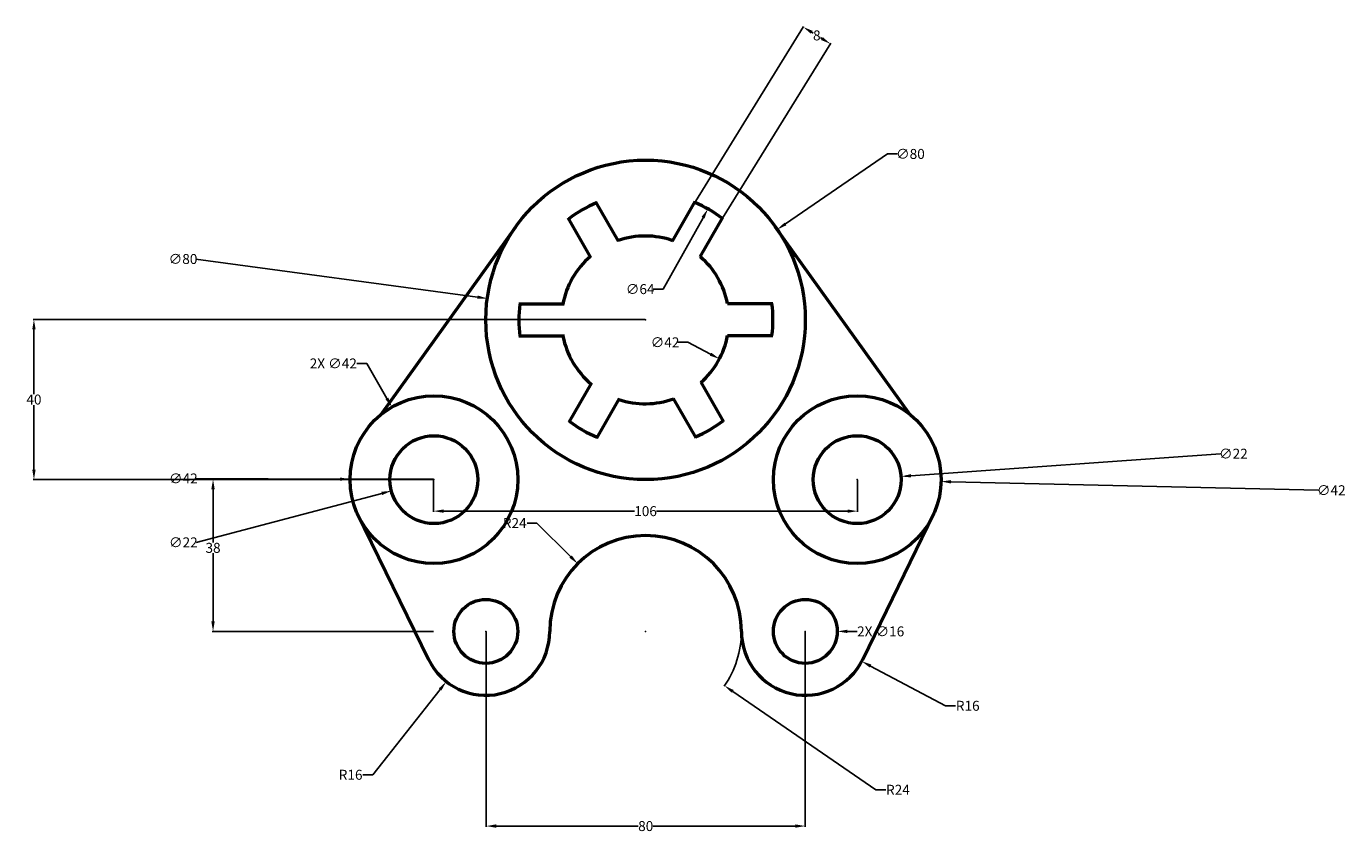
# Model space of a CAD drawing. Units: millimetres. Extents: x -109 to 221, y -17 to 185.
import ezdxf

# ---------------------------------------------------------------- set-up
doc = ezdxf.new("R2010")
doc.units = ezdxf.units.MM
doc.header["$MEASUREMENT"] = 0
doc.linetypes.add('CENTER', pattern=[50.8, 31.75, -6.35, 6.35, -6.35])
for name, color, linetype, lineweight in [('M-CNTR', 1, 'CENTER', 18), ('M-DIMS', 2, 'Continuous', 25), ('M-OUTL', 7, 'Continuous', 50)]:
    doc.layers.add(name, color=color, linetype=linetype, lineweight=lineweight)
doc.styles.get("Standard").update_dxf_attribs({"font": 'arial.ttf'})
doc.dimstyles.get("Standard").update_dxf_attribs({"dimtxt": 2.5, "dimasz": 2.5, "dimexe": 0.18, "dimexo": 0.0625, "dimgap": 0.09, "dimtad": 0, "dimtih": 1, "dimtoh": 1, "dimdec": 0, "dimzin": 0, "dimdsep": 46, "dimtxsty": 'Standard', "dimcen": 0.09, "dimadec": 0, "dimazin": 0, "dimtfac": 1, "dimtdec": 0, "dimtofl": 0, "dimtmove": 0, "dimatfit": 3, "dimfxl": 1, "dimtolj": 1, "dimtzin": 0, "dimarcsym": 0})

# ---------------------------------------------------------------- blocks, each defined once
blk = doc.blocks.new('*D1')
at = {"layer": 'Defpoints', "color": 0, "transparency": 16777216}
for p in [(5.99, 117.08), (85.26, 106.35)]:
    blk.add_point(p, dxfattribs=at)
at = {"layer": 'M-DIMS', "color": 0, "lineweight": -2, "transparency": 16777216}
for p, q in [((-66.97, 126.95), (3.51, 117.41)), ((45.54, 111.71), (45.72, 111.71)), ((45.63, 111.62), (45.63, 111.8))]:
    blk.add_line(p, q, dxfattribs=at)
at = {"layer": 'M-DIMS', "color": 0, "transparency": 16777216}
blk.add_solid([(3.57, 117.82), (3.45, 117), (5.99, 117.08)], dxfattribs=at)
at = {"layer": 'M-DIMS', "color": 0, "transparency": 16777216, "insert": (-70.2, 126.95), "char_height": 2.5, "attachment_point": 5}
blk.add_mtext('\\A1;∅80', dxfattribs=at)
blk = doc.blocks.new('*D2')
at = {"layer": 'Defpoints', "color": 0, "transparency": 16777216}
for p in [(-28.37, 71.82), (13.63, 71.61)]:
    blk.add_point(p, dxfattribs=at)
at = {"layer": 'M-DIMS', "color": 0, "lineweight": -2, "transparency": 16777216}
for p, q in [((-66.89, 72), (-30.87, 71.83)), ((-7.46, 71.71), (-7.28, 71.71)), ((-7.37, 71.62), (-7.37, 71.8))]:
    blk.add_line(p, q, dxfattribs=at)
at = {"layer": 'M-DIMS', "color": 0, "transparency": 16777216}
blk.add_solid([(-30.87, 72.24), (-30.88, 71.41), (-28.37, 71.82)], dxfattribs=at)
at = {"layer": 'M-DIMS', "color": 0, "transparency": 16777216, "insert": (-70.12, 72), "char_height": 2.5, "attachment_point": 5}
blk.add_mtext('\\A1;∅42', dxfattribs=at)
blk = doc.blocks.new('*D3')
at = {"layer": 'Defpoints', "color": 0, "transparency": 16777216}
for p in [(3.26, 74.52), (-18.01, 68.9)]:
    blk.add_point(p, dxfattribs=at)
at = {"layer": 'M-DIMS', "color": 0, "lineweight": -2, "transparency": 16777216}
for p, q in [((-7.46, 71.71), (-7.28, 71.71)), ((-7.37, 71.62), (-7.37, 71.8)), ((-66.89, 56), (-20.43, 68.27))]:
    blk.add_line(p, q, dxfattribs=at)
at = {"layer": 'M-DIMS', "color": 0, "transparency": 16777216}
blk.add_solid([(-20.53, 68.67), (-20.32, 67.86), (-18.01, 68.9)], dxfattribs=at)
at = {"layer": 'M-DIMS', "color": 0, "transparency": 16777216, "insert": (-70.12, 56), "char_height": 2.5, "attachment_point": 5}
blk.add_mtext('\\A1;∅22', dxfattribs=at)
blk = doc.blocks.new('*D4')
at = {"layer": 'Defpoints', "color": 0, "transparency": 16777216}
for p in [(77.63, 72.2), (119.62, 71.23)]:
    blk.add_point(p, dxfattribs=at)
at = {"layer": 'M-DIMS', "color": 0, "lineweight": -2, "transparency": 16777216}
for p, q in [((98.54, 71.71), (98.72, 71.71)), ((98.63, 71.62), (98.63, 71.8)), ((214.11, 69.05), (122.12, 71.17))]:
    blk.add_line(p, q, dxfattribs=at)
at = {"layer": 'M-DIMS', "color": 0, "transparency": 16777216}
blk.add_solid([(122.13, 71.59), (122.11, 70.75), (119.62, 71.23)], dxfattribs=at)
at = {"layer": 'M-DIMS', "color": 0, "transparency": 16777216, "insert": (217.34, 69.05), "char_height": 2.5, "attachment_point": 5}
blk.add_mtext('\\A1;∅42', dxfattribs=at)
blk = doc.blocks.new('*D5')
at = {"layer": 'Defpoints', "color": 0, "transparency": 16777216}
for p in [(87.65, 70.93), (109.6, 72.5)]:
    blk.add_point(p, dxfattribs=at)
at = {"layer": 'M-DIMS', "color": 0, "lineweight": -2, "transparency": 16777216}
for p, q in [((189.59, 78.2), (112.09, 72.67)), ((98.54, 71.71), (98.72, 71.71)), ((98.63, 71.62), (98.63, 71.8))]:
    blk.add_line(p, q, dxfattribs=at)
at = {"layer": 'M-DIMS', "color": 0, "transparency": 16777216}
blk.add_solid([(112.06, 73.09), (112.12, 72.26), (109.6, 72.5)], dxfattribs=at)
at = {"layer": 'M-DIMS', "color": 0, "transparency": 16777216, "insert": (192.82, 78.2), "char_height": 2.5, "attachment_point": 5}
blk.add_mtext('\\A1;∅22', dxfattribs=at)
blk = doc.blocks.new('*D6')
at = {"layer": 'Defpoints', "color": 0, "transparency": 16777216}
for p in [(45.63, 33.71), (65.4, 20.11)]:
    blk.add_point(p, dxfattribs=at)
at = {"layer": 'M-DIMS', "color": 0, "lineweight": -2, "transparency": 16777216}
for p, q in [((45.54, 33.71), (45.72, 33.71)), ((45.63, 33.62), (45.63, 33.8)), ((103.26, -5.95), (67.46, 18.69)), ((105.76, -5.95), (103.26, -5.95))]:
    blk.add_line(p, q, dxfattribs=at)
blk.add_arc((45.63, 33.71), 24, 325.0363, 359.8508, dxfattribs=at)
at = {"layer": 'M-DIMS', "color": 0, "transparency": 16777216}
blk.add_solid([(67.69, 19.03), (67.22, 18.35), (65.4, 20.11)], dxfattribs=at)
at = {"layer": 'M-DIMS', "color": 0, "transparency": 16777216, "insert": (108.83, -5.95), "char_height": 2.5, "attachment_point": 5}
blk.add_mtext('\\A1;R24', dxfattribs=at)
blk = doc.blocks.new('*D7')
at = {"layer": 'Defpoints', "color": 0, "transparency": 16777216}
for p in [(85.63, 33.71), (99.76, 26.21)]:
    blk.add_point(p, dxfattribs=at)
at = {"layer": 'M-DIMS', "color": 0, "lineweight": -2, "transparency": 16777216}
for p, q in [((85.54, 33.71), (85.72, 33.71)), ((85.63, 33.62), (85.63, 33.8)), ((120.73, 15.08), (101.97, 25.04)), ((123.23, 15.08), (120.73, 15.08))]:
    blk.add_line(p, q, dxfattribs=at)
at = {"layer": 'M-DIMS', "color": 0, "transparency": 16777216}
blk.add_solid([(102.16, 25.41), (101.77, 24.67), (99.76, 26.21)], dxfattribs=at)
at = {"layer": 'M-DIMS', "color": 0, "transparency": 16777216, "insert": (126.31, 15.08), "char_height": 2.5, "attachment_point": 5}
blk.add_mtext('\\A1;R16', dxfattribs=at)
blk = doc.blocks.new('*D8')
at = {"layer": 'Defpoints', "color": 0, "transparency": 16777216}
for p in [(5.63, 33.71), (-4.27, 21.14)]:
    blk.add_point(p, dxfattribs=at)
at = {"layer": 'M-DIMS', "color": 0, "lineweight": -2, "transparency": 16777216}
for p, q in [((5.54, 33.71), (5.72, 33.71)), ((5.63, 33.62), (5.63, 33.8)), ((-22.64, -2.19), (-5.82, 19.18)), ((-25.14, -2.19), (-22.64, -2.19))]:
    blk.add_line(p, q, dxfattribs=at)
at = {"layer": 'M-DIMS', "color": 0, "transparency": 16777216}
blk.add_solid([(-6.15, 19.43), (-5.49, 18.92), (-4.27, 21.14)], dxfattribs=at)
at = {"layer": 'M-DIMS', "color": 0, "transparency": 16777216, "insert": (-28.22, -2.19), "char_height": 2.5, "attachment_point": 5}
blk.add_mtext('\\A1;R16', dxfattribs=at)
blk = doc.blocks.new('*D9')
at = {"layer": 'Defpoints', "color": 0, "transparency": 16777216}
for p in [(5.72, 33.71), (85.63, 33.8), (85.63, -15.03)]:
    blk.add_point(p, dxfattribs=at)
at = {"layer": 'M-DIMS', "color": 0, "lineweight": -2, "transparency": 16777216}
for p, q in [((5.72, 33.65), (5.72, -15.21)), ((85.63, 33.74), (85.63, -15.21)), ((8.22, -15.03), (43.79, -15.03)), ((83.13, -15.03), (47.55, -15.03))]:
    blk.add_line(p, q, dxfattribs=at)
at = {"layer": 'M-DIMS', "color": 0, "transparency": 16777216}
for points in [[(8.22, -14.61), (8.22, -15.45), (5.72, -15.03)], [(83.13, -14.61), (83.13, -15.45), (85.63, -15.03)]]:
    blk.add_solid(points, dxfattribs=at)
at = {"layer": 'M-DIMS', "color": 0, "transparency": 16777216, "insert": (45.67, -15.03), "char_height": 2.5, "attachment_point": 5}
blk.add_mtext('\\A1;80', dxfattribs=at)
blk = doc.blocks.new('*D10')
at = {"layer": 'Defpoints', "color": 0, "transparency": 16777216}
for p in [(45.63, 111.8), (-107.53, 71.71), (-7.46, 71.71)]:
    blk.add_point(p, dxfattribs=at)
at = {"layer": 'M-DIMS', "color": 0, "lineweight": -2, "transparency": 16777216}
for p, q in [((45.56, 111.8), (-107.71, 111.8)), ((-107.53, 109.3), (-107.53, 93.12)), ((-107.53, 74.21), (-107.53, 90.39)), ((-7.53, 71.71), (-107.71, 71.71))]:
    blk.add_line(p, q, dxfattribs=at)
at = {"layer": 'M-DIMS', "color": 0, "transparency": 16777216}
for points in [[(-107.95, 109.3), (-107.11, 109.3), (-107.53, 111.8)], [(-107.95, 74.21), (-107.11, 74.21), (-107.53, 71.71)]]:
    blk.add_solid(points, dxfattribs=at)
at = {"layer": 'M-DIMS', "color": 0, "transparency": 16777216, "insert": (-107.53, 91.76), "char_height": 2.5, "attachment_point": 5}
blk.add_mtext('\\A1;40', dxfattribs=at)
blk = doc.blocks.new('*D11')
at = {"layer": 'Defpoints', "color": 0, "transparency": 16777216}
for p in [(-7.37, 71.8), (-62.68, 33.71), (-7.37, 33.71)]:
    blk.add_point(p, dxfattribs=at)
at = {"layer": 'M-DIMS', "color": 0, "lineweight": -2, "transparency": 16777216}
for p, q in [((-7.44, 71.8), (-62.86, 71.8)), ((-62.68, 69.3), (-62.68, 56)), ((-62.68, 36.21), (-62.68, 53.26)), ((-7.44, 33.71), (-62.86, 33.71))]:
    blk.add_line(p, q, dxfattribs=at)
at = {"layer": 'M-DIMS', "color": 0, "transparency": 16777216}
for points in [[(-63.1, 69.3), (-62.27, 69.3), (-62.68, 71.8)], [(-63.1, 36.21), (-62.27, 36.21), (-62.68, 33.71)]]:
    blk.add_solid(points, dxfattribs=at)
at = {"layer": 'M-DIMS', "color": 0, "transparency": 16777216, "insert": (-62.68, 54.63), "char_height": 2.5, "attachment_point": 5}
blk.add_mtext('\\A1;38', dxfattribs=at)
blk = doc.blocks.new('*D12')
at = {"layer": 'Defpoints', "color": 0, "transparency": 16777216}
for p in [(-7.46, 71.71), (98.72, 71.71), (98.72, 63.82)]:
    blk.add_point(p, dxfattribs=at)
at = {"layer": 'M-DIMS', "color": 0, "lineweight": -2, "transparency": 16777216}
for p, q in [((-7.46, 71.65), (-7.46, 63.64)), ((98.72, 71.65), (98.72, 63.64)), ((-4.96, 63.82), (42.89, 63.82)), ((96.22, 63.82), (48.36, 63.82))]:
    blk.add_line(p, q, dxfattribs=at)
at = {"layer": 'M-DIMS', "color": 0, "transparency": 16777216}
for points in [[(-4.96, 64.24), (-4.96, 63.41), (-7.46, 63.82)], [(96.22, 64.24), (96.22, 63.41), (98.72, 63.82)]]:
    blk.add_solid(points, dxfattribs=at)
at = {"layer": 'M-DIMS', "color": 0, "transparency": 16777216, "insert": (45.63, 63.82), "char_height": 2.5, "attachment_point": 5}
blk.add_mtext('\\A1;106', dxfattribs=at)
blk = doc.blocks.new('*D13')
at = {"layer": 'Defpoints', "color": 0, "transparency": 16777216}
for p in [(78.61, 134.33), (12.64, 89.09)]:
    blk.add_point(p, dxfattribs=at)
at = {"layer": 'M-DIMS', "color": 0, "lineweight": -2, "transparency": 16777216}
for p, q in [((106.22, 153.26), (80.68, 135.75)), ((108.72, 153.26), (106.22, 153.26)), ((45.54, 111.71), (45.72, 111.71)), ((45.63, 111.62), (45.63, 111.8))]:
    blk.add_line(p, q, dxfattribs=at)
at = {"layer": 'M-DIMS', "color": 0, "transparency": 16777216}
blk.add_solid([(80.44, 136.09), (80.91, 135.4), (78.61, 134.33)], dxfattribs=at)
at = {"layer": 'M-DIMS', "color": 0, "transparency": 16777216, "insert": (111.95, 153.26), "char_height": 2.5, "attachment_point": 5}
blk.add_mtext('\\A1;∅80', dxfattribs=at)
blk = doc.blocks.new('*U14')
for p, q in [((-5.7, 4), (5.7, 4)), ((-5.67, -4), (5.7, -4))]:
    blk.add_line(p, q)
blk.add_arc((-26.3, -0.09), 32, 352.9816, 7.3432)
blk = doc.blocks.new('*U15')
at = {"layer": 'M-OUTL', "color": 0, "linetype": 'ByBlock', "lineweight": -2, "transparency": 16777216}
for p, rotation in [((32.58, 134.29), 120), ((58.7, 134.38), 60), ((19.6, 111.62), 180), ((32.73, 89.05), 239.9999999999999), ((58.85, 89.14), 299.9999999999999)]:
    blk.add_blockref('*U14', p, dxfattribs=dict(at, rotation=rotation))
blk.add_blockref('*U14', (71.83, 111.8), dxfattribs=at)
blk = doc.blocks.new('*D16')
at = {"layer": 'Defpoints', "color": 0, "transparency": 16777216}
for p in [(91.91, 180.83), (58.08, 141.31), (64.89, 137.11)]:
    blk.add_point(p, dxfattribs=at)
at = {"layer": 'M-DIMS', "color": 0, "lineweight": -2, "transparency": 16777216}
for p, q in [((58.12, 141.37), (85.2, 185.19)), ((87.23, 183.73), (87.6, 183.5)), ((89.79, 182.15), (89.42, 182.37)), ((64.92, 137.16), (92.01, 180.99))]:
    blk.add_line(p, q, dxfattribs=at)
at = {"layer": 'M-DIMS', "color": 0, "transparency": 16777216}
for points in [[(87.45, 184.08), (87.01, 183.37), (85.11, 185.04)], [(90.01, 182.5), (89.57, 181.79), (91.91, 180.83)]]:
    blk.add_solid(points, dxfattribs=at)
at = {"layer": 'M-DIMS', "color": 0, "transparency": 16777216, "insert": (88.51, 182.94), "char_height": 2.5, "attachment_point": 5}
blk.add_mtext('\\A1;8', dxfattribs=at)
blk = doc.blocks.new('*D17')
at = {"layer": 'Defpoints', "color": 0, "transparency": 16777216}
for p in [(26.94, 121.48), (64.13, 101.95)]:
    blk.add_point(p, dxfattribs=at)
at = {"layer": 'M-DIMS', "color": 0, "lineweight": -2, "transparency": 16777216}
for p, q in [((53.74, 106.09), (56.24, 106.09)), ((56.24, 106.09), (61.91, 103.11))]:
    blk.add_line(p, q, dxfattribs=at)
at = {"layer": 'M-DIMS', "color": 0, "transparency": 16777216}
blk.add_solid([(62.11, 103.48), (61.72, 102.74), (64.13, 101.95)], dxfattribs=at)
at = {"layer": 'M-DIMS', "color": 0, "transparency": 16777216, "insert": (50.51, 106.09), "char_height": 2.5, "attachment_point": 5}
blk.add_mtext('\\A1;∅42', dxfattribs=at)
blk = doc.blocks.new('*D18')
at = {"layer": 'Defpoints', "color": 0, "transparency": 16777216}
for p in [(61.24, 139.49), (30.01, 83.63)]:
    blk.add_point(p, dxfattribs=at)
at = {"layer": 'M-DIMS', "color": 0, "lineweight": -2, "transparency": 16777216}
for p, q in [((50.02, 119.41), (60.02, 137.3)), ((47.52, 119.41), (50.02, 119.41))]:
    blk.add_line(p, q, dxfattribs=at)
at = {"layer": 'M-DIMS', "color": 0, "transparency": 16777216}
blk.add_solid([(59.66, 137.51), (60.39, 137.1), (61.24, 139.49)], dxfattribs=at)
at = {"layer": 'M-DIMS', "color": 0, "transparency": 16777216, "insert": (44.28, 119.41), "char_height": 2.5, "attachment_point": 5}
blk.add_mtext('\\A1;∅64', dxfattribs=at)
blk = doc.blocks.new('*D19')
at = {"layer": 'Defpoints', "color": 0, "transparency": 16777216}
for p in [(-17.89, 89.89), (3.14, 53.54)]:
    blk.add_point(p, dxfattribs=at)
at = {"layer": 'M-DIMS', "color": 0, "lineweight": -2, "transparency": 16777216}
for p, q in [((-26.7, 100.79), (-24.2, 100.79)), ((-24.2, 100.79), (-19.15, 92.05)), ((-7.46, 71.71), (-7.28, 71.71)), ((-7.37, 71.62), (-7.37, 71.8))]:
    blk.add_line(p, q, dxfattribs=at)
at = {"layer": 'M-DIMS', "color": 0, "transparency": 16777216}
blk.add_solid([(-18.78, 92.26), (-19.51, 91.84), (-17.89, 89.89)], dxfattribs=at)
at = {"layer": 'M-DIMS', "color": 0, "transparency": 16777216, "insert": (-32.57, 100.79), "char_height": 2.5, "attachment_point": 5}
blk.add_mtext('\\A1;2X ∅42', dxfattribs=at)
blk = doc.blocks.new('*D20')
at = {"layer": 'Defpoints', "color": 0, "transparency": 16777216}
for p in [(77.63, 33.71), (93.63, 33.71)]:
    blk.add_point(p, dxfattribs=at)
at = {"layer": 'M-DIMS', "color": 0, "lineweight": -2, "transparency": 16777216}
for p, q in [((85.54, 33.71), (85.72, 33.71)), ((85.63, 33.62), (85.63, 33.8)), ((98.63, 33.71), (96.13, 33.71))]:
    blk.add_line(p, q, dxfattribs=at)
at = {"layer": 'M-DIMS', "color": 0, "transparency": 16777216}
blk.add_solid([(96.13, 34.13), (96.13, 33.3), (93.63, 33.71)], dxfattribs=at)
at = {"layer": 'M-DIMS', "color": 0, "transparency": 16777216, "insert": (104.51, 33.71), "char_height": 2.5, "attachment_point": 5}
blk.add_mtext('\\A1;2X ∅16', dxfattribs=at)
blk = doc.blocks.new('*D21')
at = {"layer": 'Defpoints', "color": 0, "transparency": 16777216}
for p in [(28.64, 50.66), (45.63, 33.71)]:
    blk.add_point(p, dxfattribs=at)
at = {"layer": 'M-DIMS', "color": 0, "lineweight": -2, "transparency": 16777216}
for p, q in [((15.94, 60.83), (18.44, 60.83)), ((18.44, 60.83), (26.87, 52.43)), ((45.54, 33.71), (45.72, 33.71)), ((45.63, 33.62), (45.63, 33.8))]:
    blk.add_line(p, q, dxfattribs=at)
at = {"layer": 'M-DIMS', "color": 0, "transparency": 16777216}
blk.add_solid([(27.16, 52.72), (26.57, 52.13), (28.64, 50.66)], dxfattribs=at)
at = {"layer": 'M-DIMS', "color": 0, "transparency": 16777216, "insert": (12.87, 60.83), "char_height": 2.5, "attachment_point": 5}
blk.add_mtext('\\A1;R24', dxfattribs=at)

msp = doc.modelspace()

# ---------------------------------------------------------------- linework, layer by layer
at = {"layer": 'M-CNTR'}
for p in [(45.63, 111.8), (45.72, 111.71), (45.54, 111.71), (45.72, 111.71), (45.72, 111.71), (45.54, 111.71), (45.54, 111.71), (45.54, 111.71), (45.54, 111.71), (45.54, 111.71), (45.72, 111.71)]:
    msp.add_line(p, (45.54, 111.71), dxfattribs=at)
at = {"layer": 'M-OUTL'}
for p, q in [((-20.67, 87.97), (13.13, 135.04)), ((13.13, 135.04), (13.13, 135.04)), ((111.92, 87.97), (78.12, 135.04)), ((-26.58, 63.22), (-8.75, 26.69)), ((117.83, 63.22), (100, 26.69))]:
    msp.add_line(p, q, dxfattribs=at)
for centre, radius in [((45.63, 111.71), 40), ((-7.37, 71.71), 21), ((98.63, 71.71), 21), ((-7.37, 71.71), 11), ((98.63, 71.71), 11), ((5.63, 33.71), 8), ((85.63, 33.71), 8)]:
    msp.add_circle(centre, radius, dxfattribs=at)
for centre, radius, start, end in [((45.54, 111.71), 21, 70.7975, 108.8363), ((45.54, 111.71), 21, 130.7975, 169.2695), ((45.54, 111.71), 21, 11.2308, 48.8363), ((45.54, 111.71), 21, 191.2308, 229.702), ((45.54, 111.71), 21, 311.6648, 349.2695), ((45.54, 111.71), 21, 251.6648, 289.702), ((45.63, 33.71), 24, 0, 180), ((5.63, 33.71), 16, 206.016, 0), ((85.63, 33.71), 16, 180, 333.984)]:
    msp.add_arc(centre, radius, start, end, dxfattribs=at)

# ---------------------------------------------------------------- block references
msp.add_blockref('*U15', (0, 0), dxfattribs=at)

# ---------------------------------------------------------------- dimensions: what is measured, and where the dimension line sits
at = {"layer": 'M-DIMS'}
dim = msp.add_aligned_dim(p1=(58.08, 141.31), p2=(64.89, 137.11), distance=51.4, dimstyle='Standard', override={"dimclrd": 0, "dimclre": 0, "dimclrt": 0}, dxfattribs=at)
dim.commit()
dim.dimension.update_dxf_attribs({"geometry": '*D16', "text_midpoint": (88.51, 182.94)})
for p1, p2, picture, middle in [((12.64, 89.09), (78.61, 134.33), '*D13', (111.95, 153.26)), ((30.01, 83.63), (61.24, 139.49), '*D18', (44.28, 119.41)), ((85.26, 106.35), (5.99, 117.08), '*D1', (-66.97, 126.95)), ((26.94, 121.48), (64.13, 101.95), '*D17', (50.51, 106.09)), ((87.65, 70.93), (109.6, 72.5), '*D5', (189.59, 78.2)), ((3.26, 74.52), (-18.01, 68.9), '*D3', (-66.89, 56)), ((13.63, 71.61), (-28.37, 71.82), '*D2', (-66.89, 72)), ((77.63, 72.2), (119.62, 71.23), '*D4', (214.11, 69.05))]:
    dim = msp.add_diameter_dim_2p(p1=p1, p2=p2, dimstyle='Standard', override={"dimclrd": 0, "dimclre": 0, "dimclrt": 0}, dxfattribs=at)
    dim.commit()
    dim.dimension.update_dxf_attribs({"geometry": picture, "text_midpoint": middle, "dimtype": 163})
dim = msp.add_linear_dim(base=(-107.53, 71.71), p1=(45.63, 111.8), p2=(-7.46, 71.71), angle=90, dimstyle='Standard', override={"dimclrd": 0, "dimclre": 0, "dimclrt": 0}, dxfattribs=at)
dim.commit()
dim.dimension.update_dxf_attribs({"geometry": '*D10', "text_midpoint": (-107.53, 91.76)})
for p1, p2, picture, middle in [((3.14, 53.54), (-17.89, 89.89), '*D19', (-32.57, 100.79)), ((77.63, 33.71), (93.63, 33.71), '*D20', (98.63, 33.71))]:
    dim = msp.add_diameter_dim_2p(p1=p1, p2=p2, text='2X <>', dimstyle='Standard', override={"dimdec": 0, "dimlfac": 1, "dimrnd": 0, "dimzin": 0, "dimdsep": 46, "dimlunit": 2}, dxfattribs=at)
    dim.commit()
    dim.dimension.update_dxf_attribs({"geometry": picture, "text_midpoint": middle, "dimtype": 163})
dim = msp.add_linear_dim(base=(-62.68, 33.71), p1=(-7.37, 71.8), p2=(-7.37, 33.71), angle=90, dimstyle='Standard', override={"dimclrd": 0, "dimclre": 0, "dimclrt": 0}, dxfattribs=at)
dim.commit()
dim.dimension.update_dxf_attribs({"geometry": '*D11', "text_midpoint": (-62.68, 54.63), "dimtype": 160})
for base, p1, p2, picture, middle in [((98.72, 63.82), (-7.46, 71.71), (98.72, 71.71), '*D12', (45.63, 63.82)), ((85.63, -15.03), (5.72, 33.71), (85.63, 33.8), '*D9', (45.67, -15.03))]:
    dim = msp.add_linear_dim(base=base, p1=p1, p2=p2, dimstyle='Standard', override={"dimclrd": 0, "dimclre": 0, "dimclrt": 0}, dxfattribs=at)
    dim.commit()
    dim.dimension.update_dxf_attribs({"geometry": picture, "text_midpoint": middle})
for center, mpoint, override, picture, middle in [((45.63, 33.71), (28.64, 50.66), {"dimdec": 0, "dimlfac": 1, "dimrnd": 0, "dimzin": 0, "dimdsep": 46, "dimlunit": 2}, '*D21', (12.87, 60.83)), ((5.63, 33.71), (-4.27, 21.14), {"dimclrd": 0, "dimclre": 0, "dimclrt": 0}, '*D8', (-28.22, -2.19)), ((45.63, 33.71), (65.4, 20.11), {"dimclrd": 0, "dimclre": 0, "dimclrt": 0}, '*D6', (108.83, -5.95)), ((85.63, 33.71), (99.76, 26.21), {"dimclrd": 0, "dimclre": 0, "dimclrt": 0}, '*D7', (126.31, 15.08))]:
    dim = msp.add_radius_dim(center=center, mpoint=mpoint, dimstyle='Standard', override=override, dxfattribs=at)
    dim.commit()
    dim.dimension.update_dxf_attribs({"geometry": picture, "text_midpoint": middle, "dimtype": 164})

doc.saveas('drawing.dxf')
